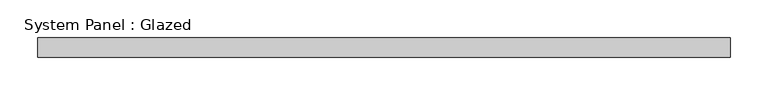
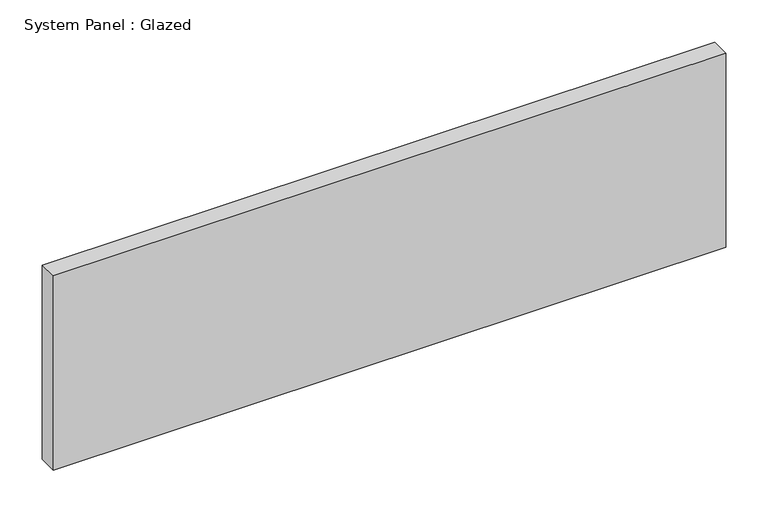
"""IFC4 building model written with IfcOpenShell, lengths in millimetres: plate geometry, System Panel : Glazed."""

from ifc_helpers import new_model, si_unit, origin, origin_with_axes, place, context, project, spatial, polyline, outline, extrude, source, transform, mapped, element, save


def system_panel_glazed_23092caa(model_context):
    return source(origin(), model_context, "Body", "SweptSolid", [
        extrude(outline(polyline([(457.2, 19.05), (-457.2, 19.05), (-457.2, 44.45), (457.2, 44.45), (457.2, 19.05)])), origin_with_axes(), (0.0, 0.0, 1.0), 279.4),
    ])


if __name__ == "__main__":
    model = new_model("IFC4")
    model_context = context("Model", 3, world=origin())
    ifc_project = project(units=[si_unit("LENGTHUNIT", "METRE", prefix="MILLI")], contexts=[model_context])
    site = spatial("IfcSite", under=ifc_project)
    building = spatial("IfcBuilding", under=site)
    placement = place(None, origin())
    system_panel_glazed_shape = system_panel_glazed_23092caa(model_context)
    element("IfcPlate", 1, ObjectType="System Panel : Glazed", at=placement, inside=building, context=model_context, shape_type="MappedRepresentation", body=[
        mapped(system_panel_glazed_shape, transform((0.0, 0.0, 0.0), x_axis=(1.0, 0.0, 0.0), y_axis=(0.0, 1.0, 0.0), z_axis=(0.0, 0.0, 1.0))),
    ])
    save(model, "model.ifc")

# Revit data of these elements
# Type "System Panel : Glazed"
#   Construction Type Id = "GSP4R"
#   Analytic Construction = "1/8 in Pilkington single glazing"
#   Visual Light Transmittance = 0.9
#   Solar Heat Gain Coefficient = 0.86
#   Heat Transfer Coefficient (U) = 1.18115 BTU/(h·ft²·°F)
#   Define Thermal Properties by = 1
# Element 1 (IfcPlate, "System Panel : Glazed")
#   Materials on its faces: "Glass"
# Materials
#   "Glass": class "Glass", colour RGB 0 128 192, transparency 0.75, Description = "Soda Lime Glass", Cost = 0
